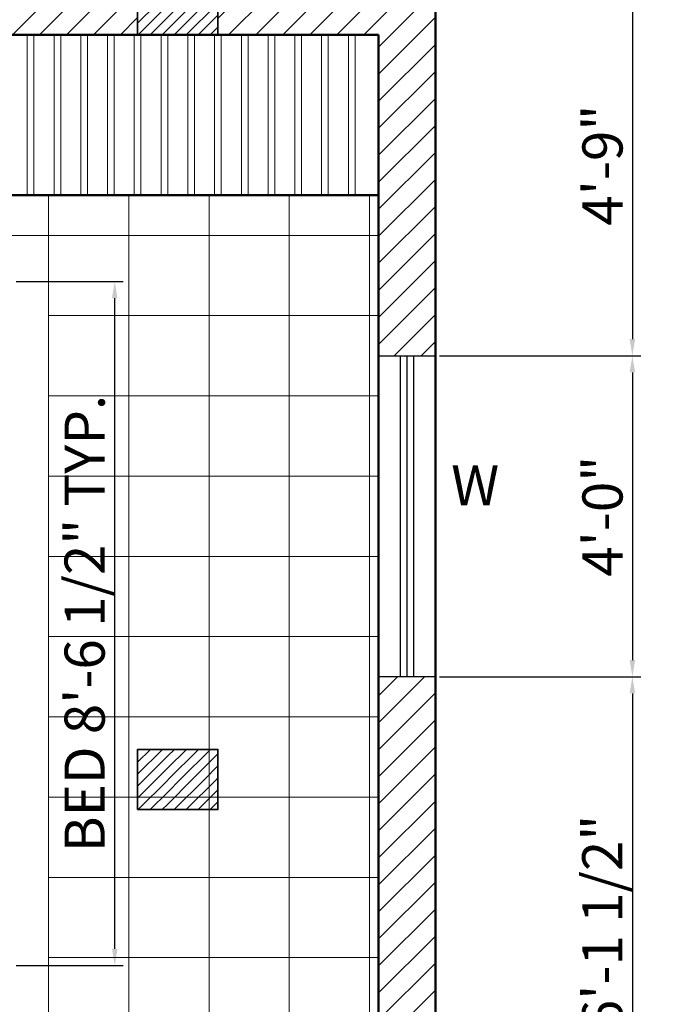
# Model space of a CAD drawing. Units: millimetres. Extents: x 225995 to 227247, y 225507 to 226008.
# Tile 22 of 23: x 227150 to 227247, y 225781 to 225928. Entities that reach past the tile are written whole.
import ezdxf

# ---------------------------------------------------------------- set-up
doc = ezdxf.new("R2010")
doc.units = ezdxf.units.MM
for name, color, linetype, lineweight in [('A-ANNO-DIMS', 2, 'Continuous', 18), ('A-ANNO-TEXT', 3, 'Continuous', 18), ('A-COLS', 40, 'Continuous', 35), ('A-FLOR-PATT', 8, 'Continuous', 13), ('A-FURN', 9, 'Continuous', 18), ('A-GLAZ', 4, 'Continuous', 25), ('A-WALL', 7, 'Continuous', 50), ('A-WALL-PATT', 8, 'Continuous', 13)]:
    doc.layers.add(name, color=color, linetype=linetype, lineweight=lineweight)
doc.styles.get("Standard").update_dxf_attribs({"font": 'arial.ttf'})
doc.dimstyles.new('ISO-25', dxfattribs={"dimtxt": 6, "dimasz": 2.5, "dimexe": 1.25, "dimexo": 0.625, "dimtad": 1, "dimdec": 0, "dimlunit": 3, "dimtxsty": 'Standard', "dimcen": 2.5, "dimadec": 0, "dimazin": 0, "dimtfac": 1, "dimtdec": 0, "dimtmove": 0, "dimatfit": 3, "dimfxl": 1, "dimarcsym": 0})
pattern_1 = [(45, (646.0463, 0.931), (-2.020557627, 2.020557627), [])]
pattern_2 = [(45, (787.0463, 119.0672), (-0.898025612, 0.898025612), [])]
pattern_3 = [(45, (787.0463, 234.931), (-0.898025612, 0.898025612), [])]

# ---------------------------------------------------------------- blocks, each defined once
blk = doc.blocks.new('*D79')
at = {"layer": 'A-ANNO-DIMS', "color": 0, "lineweight": -2, "transparency": 16777216}
for p, q in [((227149.28, 225888.79), (227165.25, 225888.79)), ((227164, 225789.02), (227164, 225886.29)), ((227149.28, 225786.52), (227165.25, 225786.52))]:
    blk.add_line(p, q, dxfattribs=at)
at = {"layer": 'A-ANNO-DIMS', "color": 0, "transparency": 16777216}
for points in [[(227163.58, 225886.29), (227164.41, 225886.29), (227164, 225888.79)], [(227163.58, 225789.02), (227164.41, 225789.02), (227164, 225786.52)]]:
    blk.add_solid(points, dxfattribs=at)
at = {"layer": 'Defpoints', "color": 0, "transparency": 16777216}
for p in [(227148.66, 225888.79), (227164, 225888.79), (227148.66, 225786.52)]:
    blk.add_point(p, dxfattribs=at)
at = {"layer": 'A-ANNO-DIMS', "color": 0, "transparency": 16777216, "insert": (227160.27, 225837.65), "char_height": 6, "attachment_point": 5, "rotation": 90}
blk.add_mtext('BED 8\'-6 1/2" TYP.', dxfattribs=at)
blk = doc.blocks.new('*D124')
at = {"layer": 'A-ANNO-DIMS', "color": 0, "lineweight": -2, "transparency": 16777216}
for p, q in [((227212.55, 225934.7), (227242.62, 225934.7)), ((227241.37, 225932.2), (227241.37, 225880.2)), ((227212.55, 225877.7), (227242.62, 225877.7))]:
    blk.add_line(p, q, dxfattribs=at)
at = {"layer": 'A-ANNO-DIMS', "color": 0, "transparency": 16777216}
for points in [[(227240.96, 225932.2), (227241.79, 225932.2), (227241.37, 225934.7)], [(227240.96, 225880.2), (227241.79, 225880.2), (227241.37, 225877.7)]]:
    blk.add_solid(points, dxfattribs=at)
at = {"layer": 'Defpoints', "color": 0, "transparency": 16777216}
for p in [(227211.92, 225934.7), (227211.92, 225877.7), (227241.37, 225877.7)]:
    blk.add_point(p, dxfattribs=at)
at = {"layer": 'A-ANNO-DIMS', "color": 0, "transparency": 16777216, "insert": (227237.68, 225906.2), "char_height": 6, "attachment_point": 5, "rotation": 90}
blk.add_mtext('4\'-9"', dxfattribs=at)
blk = doc.blocks.new('*D125')
at = {"layer": 'A-ANNO-DIMS', "color": 0, "lineweight": -2, "transparency": 16777216}
for p, q in [((227212.55, 225877.7), (227242.62, 225877.7)), ((227241.37, 225875.2), (227241.37, 225832.2)), ((227212.55, 225829.7), (227242.62, 225829.7))]:
    blk.add_line(p, q, dxfattribs=at)
at = {"layer": 'A-ANNO-DIMS', "color": 0, "transparency": 16777216}
for points in [[(227240.96, 225875.2), (227241.79, 225875.2), (227241.37, 225877.7)], [(227240.96, 225832.2), (227241.79, 225832.2), (227241.37, 225829.7)]]:
    blk.add_solid(points, dxfattribs=at)
at = {"layer": 'Defpoints', "color": 0, "transparency": 16777216}
for p in [(227211.92, 225877.7), (227211.92, 225829.7), (227241.37, 225829.7)]:
    blk.add_point(p, dxfattribs=at)
at = {"layer": 'A-ANNO-DIMS', "color": 0, "transparency": 16777216, "insert": (227237.68, 225853.7), "char_height": 6, "attachment_point": 5, "rotation": 90}
blk.add_mtext('4\'-0"', dxfattribs=at)
blk = doc.blocks.new('*D126')
at = {"layer": 'A-ANNO-DIMS', "color": 0, "lineweight": -2, "transparency": 16777216}
for p, q in [((227212.55, 225829.7), (227242.62, 225829.7)), ((227241.37, 225827.2), (227241.37, 225758.7)), ((227212.55, 225756.2), (227242.62, 225756.2))]:
    blk.add_line(p, q, dxfattribs=at)
at = {"layer": 'A-ANNO-DIMS', "color": 0, "transparency": 16777216}
for points in [[(227240.96, 225827.2), (227241.79, 225827.2), (227241.37, 225829.7)], [(227240.96, 225758.7), (227241.79, 225758.7), (227241.37, 225756.2)]]:
    blk.add_solid(points, dxfattribs=at)
at = {"layer": 'Defpoints', "color": 0, "transparency": 16777216}
for p in [(227211.92, 225829.7), (227211.92, 225756.2), (227241.37, 225756.2)]:
    blk.add_point(p, dxfattribs=at)
at = {"layer": 'A-ANNO-DIMS', "color": 0, "transparency": 16777216, "insert": (227237.65, 225792.95), "char_height": 6, "attachment_point": 5, "rotation": 90}
blk.add_mtext('6\'-1 1/2"', dxfattribs=at)

msp = doc.modelspace()

# ---------------------------------------------------------------- hatches: boundary and pattern name
at = {"layer": 'A-WALL-PATT'}
h = msp.add_hatch(dxfattribs=at)
h.set_pattern_fill('ANSI31', color=256, scale=0.9)
h.set_pattern_definition(pattern_1)
h.paths.add_polyline_path([(227167.42, 225934.7), (227038.42, 225934.7), (227038.42, 225925.7), (227167.42, 225925.7)])
h = msp.add_hatch(dxfattribs=at)
h.set_pattern_fill('ANSI31', color=256, scale=0.9)
h.set_pattern_definition(pattern_1)
h.paths.add_polyline_path([(227211.92, 225934.7), (227179.42, 225934.7), (227179.42, 225925.7), (227203.42, 225925.7), (227203.42, 225877.7), (227211.92, 225877.7)])
h = msp.add_hatch(dxfattribs=at)
h.set_pattern_fill('ANSI31', color=256, scale=0.4)
h.set_pattern_definition(pattern_3)
h.paths.add_polyline_path([(227171.92, 225930.2), (227167.42, 225930.2), (227167.42, 225925.7), (227171.92, 225925.7)])
h = msp.add_hatch(dxfattribs=at)
h.set_pattern_fill('ANSI31', color=256, scale=0.4)
h.set_pattern_definition(pattern_3)
h.paths.add_polyline_path([(227179.42, 225930.2), (227171.92, 225930.2), (227171.92, 225925.7), (227179.42, 225925.7)])
h = msp.add_hatch(dxfattribs=at)
h.set_pattern_fill('ANSI31', color=256, scale=0.9)
h.set_pattern_definition(pattern_1)
h.paths.add_polyline_path([(227211.92, 225829.7), (227203.42, 225829.7), (227203.42, 225756.2), (227211.92, 225756.2)])
h = msp.add_hatch(dxfattribs=at)
h.set_pattern_fill('ANSI31', color=256, scale=0.4)
h.set_pattern_definition(pattern_2)
h.paths.add_polyline_path([(227171.92, 225818.84), (227167.42, 225818.84), (227167.42, 225814.34), (227171.92, 225814.34)])
h = msp.add_hatch(dxfattribs=at)
h.set_pattern_fill('ANSI31', color=256, scale=0.4)
h.set_pattern_definition(pattern_2)
h.paths.add_polyline_path([(227179.42, 225818.84), (227171.92, 225818.84), (227171.92, 225814.34), (227179.42, 225814.34)])
h = msp.add_hatch(dxfattribs=at)
h.set_pattern_fill('ANSI31', color=256, scale=0.4)
h.set_pattern_definition(pattern_2)
h.paths.add_polyline_path([(227171.92, 225814.34), (227167.42, 225814.34), (227167.42, 225809.84), (227171.92, 225809.84)])
h = msp.add_hatch(dxfattribs=at)
h.set_pattern_fill('ANSI31', color=256, scale=0.4)
h.set_pattern_definition(pattern_2)
h.paths.add_polyline_path([(227179.42, 225814.34), (227171.92, 225814.34), (227171.92, 225809.84), (227179.42, 225809.84)])

# ---------------------------------------------------------------- linework, layer by layer
at = {"layer": 'A-COLS'}
for points in [[(227167.42, 225925.7), (227167.42, 225934.7), (227179.42, 225934.7), (227179.42, 225925.7)], [(227167.42, 225809.84), (227167.42, 225818.84), (227179.42, 225818.84), (227179.42, 225809.84)]]:
    msp.add_lwpolyline(points, close=True, dxfattribs=at)
at = {"layer": 'A-FLOR-PATT'}
for p, q in [((227154.09, 225901.7), (227154.09, 225696.2)), ((227166.09, 225901.7), (227166.09, 225696.2)), ((227178.09, 225901.7), (227178.09, 225700.7)), ((227190.09, 225901.7), (227190.09, 225696.2)), ((227030.92, 225895.7), (227203.42, 225895.7)), ((227154.09, 225883.7), (227203.42, 225883.7)), ((227154.09, 225871.7), (227203.42, 225871.7)), ((227154.09, 225859.7), (227203.42, 225859.7)), ((227154.09, 225847.7), (227203.42, 225847.7)), ((227154.09, 225835.7), (227203.42, 225835.7)), ((227154.09, 225823.7), (227203.42, 225823.7)), ((227154.09, 225811.7), (227203.42, 225811.7)), ((227154.09, 225799.7), (227203.42, 225799.7)), ((227154.09, 225787.7), (227203.42, 225787.7))]:
    msp.add_line(p, q, dxfattribs=at)
at = {"layer": 'A-FURN'}
for p, q in [((227150.92, 225901.7), (227150.92, 225925.7)), ((227151.92, 225901.7), (227151.92, 225925.7)), ((227154.92, 225901.7), (227154.92, 225925.7)), ((227155.92, 225901.7), (227155.92, 225925.7)), ((227158.92, 225901.7), (227158.92, 225925.7)), ((227159.92, 225901.7), (227159.92, 225925.7)), ((227162.92, 225901.7), (227162.92, 225925.7)), ((227163.92, 225901.7), (227163.92, 225925.7)), ((227166.92, 225901.7), (227166.92, 225925.7)), ((227167.92, 225901.7), (227167.92, 225925.7)), ((227170.92, 225901.7), (227170.92, 225925.7)), ((227171.92, 225901.7), (227171.92, 225925.7)), ((227174.92, 225901.7), (227174.92, 225925.7)), ((227175.92, 225901.7), (227175.92, 225925.7)), ((227178.92, 225901.7), (227178.92, 225925.7)), ((227179.92, 225901.7), (227179.92, 225925.7)), ((227182.92, 225901.7), (227182.92, 225925.7)), ((227183.92, 225901.7), (227183.92, 225925.7)), ((227186.92, 225901.7), (227186.92, 225925.7)), ((227187.92, 225901.7), (227187.92, 225925.7)), ((227190.92, 225901.7), (227190.92, 225925.7)), ((227191.92, 225901.7), (227191.92, 225925.7)), ((227194.92, 225901.7), (227194.92, 225925.7)), ((227195.92, 225901.7), (227195.92, 225925.7)), ((227198.92, 225901.7), (227198.92, 225925.7)), ((227199.92, 225901.7), (227199.92, 225925.7)), ((227202.09, 225901.7), (227202.09, 225696.2)), ((227203.42, 225877.7), (227211.92, 225877.7)), ((227203.42, 225829.7), (227211.92, 225829.7))]:
    msp.add_line(p, q, dxfattribs=at)
at = {"layer": 'A-GLAZ'}
for p, q in [((227206.67, 225877.7), (227206.67, 225829.7)), ((227207.67, 225877.7), (227207.67, 225829.7)), ((227208.67, 225877.7), (227208.67, 225829.7))]:
    msp.add_line(p, q, dxfattribs=at)
msp.add_lwpolyline([(227203.42, 225877.7), (227211.92, 225877.7), (227211.92, 225829.7), (227203.42, 225829.7)], close=True, dxfattribs=at)
at = {"layer": 'A-WALL'}
for p, q in [((227211.92, 225934.7), (227211.92, 225571.7)), ((227211.92, 225934.7), (227211.92, 225571.7)), ((227030.92, 225925.7), (227203.42, 225925.7)), ((227203.42, 225925.7), (227030.92, 225925.7)), ((227203.42, 225696.2), (227203.42, 225925.7)), ((227203.42, 225696.2), (227203.42, 225925.7)), ((227030.92, 225901.7), (227203.42, 225901.7))]:
    msp.add_line(p, q, dxfattribs=at)

# ---------------------------------------------------------------- texts
at = {"layer": 'A-ANNO-TEXT', "insert": (227208.78, 225861.32), "char_height": 6, "attachment_point": 1}
msp.add_mtext_dynamic_manual_height_columns('   W', width=24.8115, gutter_width=12.5, heights=[0], dxfattribs=at)

# ---------------------------------------------------------------- dimensions: what is measured, and where the dimension line sits
at = {"layer": 'A-ANNO-DIMS'}
for base, p1, p2, picture, middle in [((227241.37, 225877.7), (227211.92, 225934.7), (227211.92, 225877.7), '*D124', (227237.68, 225906.2)), ((227241.37, 225829.7), (227211.92, 225877.7), (227211.92, 225829.7), '*D125', (227237.68, 225853.7)), ((227241.37, 225756.2), (227211.92, 225829.7), (227211.92, 225756.2), '*D126', (227237.65, 225792.95))]:
    dim = msp.add_linear_dim(base=base, p1=p1, p2=p2, angle=90, dimstyle='ISO-25', override={"dimdec": 1, "dimlfac": 1, "dimrnd": 0, "dimzin": 1, "dimdsep": 46, "dimlunit": 4, "dimfrac": 2}, dxfattribs=at)
    dim.commit()
    dim.dimension.update_dxf_attribs({"geometry": picture, "text_midpoint": middle})
dim = msp.add_linear_dim(base=(227164, 225888.79), p1=(227148.66, 225786.52), p2=(227148.66, 225888.79), angle=90, text='BED <> TYP.', dimstyle='ISO-25', override={"dimdec": 1, "dimrnd": 0, "dimzin": 1, "dimlunit": 4, "dimfrac": 2}, dxfattribs=at)
dim.commit()
dim.dimension.update_dxf_attribs({"geometry": '*D79', "text_midpoint": (227160.27, 225837.65)})

doc.saveas('drawing.dxf')
